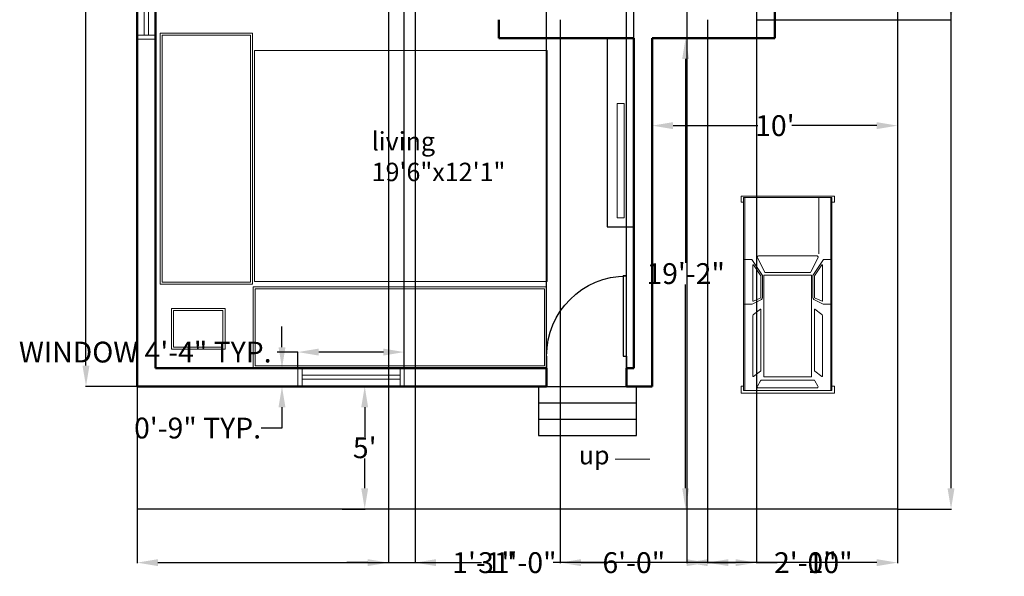
# Model space of a CAD drawing. Units: inches. Extents: x 20 to 3619, y 7 to 1288.
# Tile 1 of 4: x 3085 to 3567, y 695 to 967. Entities that reach past the tile are written whole.
import ezdxf

# ---------------------------------------------------------------- set-up
doc = ezdxf.new("R2010")
doc.units = ezdxf.units.IN
doc.header["$MEASUREMENT"] = 0
for name, color, linetype, lineweight in [('A-ANNO-DIMS', 2, 'Continuous', 18), ('A-ANNO-SYMB', 7, 'Continuous', 18), ('A-ANNO-TEXT', 7, 'Continuous', 18), ('A-AREA-IDEN', 7, 'Continuous', 25), ('A-DOOR', 3, 'Continuous', 25), ('A-FLOR-CASE', 9, 'Continuous', 25), ('A-FLOR-STRS', 7, 'Continuous', 25), ('A-FURN', 8, 'Continuous', 18), ('A-GLAZ', 4, 'Continuous', 18), ('A-SITE-VEHC', 8, 'Continuous', 13), ('A-WALL', 7, 'Continuous', 50), ('C-PROP', 8, 'Continuous', 25)]:
    doc.layers.add(name, color=color, linetype=linetype, lineweight=lineweight)
doc.styles.get("Standard").update_dxf_attribs({"font": 'arial.ttf'})
doc.dimstyles.get("Standard").update_dxf_attribs({"dimtxt": 10.18, "dimasz": 10.18, "dimexe": 0.18, "dimexo": 0.0625, "dimgap": 0.09, "dimtad": 0, "dimtih": 1, "dimtoh": 1, "dimdec": 0, "dimzin": 0, "dimdsep": 46, "dimlunit": 3, "dimtxsty": 'Standard', "dimcen": 0.09, "dimadec": 0, "dimazin": 0, "dimtfac": 1, "dimtdec": 0, "dimtofl": 0, "dimtmove": 0, "dimatfit": 3, "dimfxl": 1, "dimtolj": 1, "dimtzin": 0, "dimarcsym": 0})

# ---------------------------------------------------------------- blocks, each defined once
blk = doc.blocks.new('*U2')
for p, q in [((0, 0), (0, -6)), ((40, 0), (40, -6))]:
    blk.add_line(p, q)
blk.add_lwpolyline([(0, 0), (0, 40), (1.75, 40), (1.75, 0)], close=True)
blk.add_arc((0, 0), 40, 0, 90)
blk = doc.blocks.new('*D4')
at = {"layer": 'A-ANNO-DIMS', "color": 0, "lineweight": -2, "transparency": 16777216}
for p, q in [((3142.66, 1195.69), (3117.53, 1195.69)), ((3117.71, 1185.51), (3117.71, 996.98)), ((3117.71, 797.87), (3117.71, 986.4)), ((3142.66, 787.69), (3117.53, 787.69))]:
    blk.add_line(p, q, dxfattribs=at)
at = {"layer": 'A-ANNO-DIMS', "color": 0, "transparency": 16777216}
for points in [[(3116.01, 1185.51), (3119.4, 1185.51), (3117.71, 1195.69)], [(3116.01, 797.87), (3119.4, 797.87), (3117.71, 787.69)]]:
    blk.add_solid(points, dxfattribs=at)
at = {"layer": 'Defpoints', "color": 0, "transparency": 16777216}
for p in [(3117.71, 1195.69), (3142.72, 1195.69), (3142.72, 787.69)]:
    blk.add_point(p, dxfattribs=at)
at = {"layer": 'A-ANNO-DIMS', "color": 0, "transparency": 16777216, "insert": (3117.71, 991.69), "char_height": 10.18, "attachment_point": 5}
blk.add_mtext("\\A1;34'", dxfattribs=at)
blk = doc.blocks.new('*D6')
at = {"layer": 'A-ANNO-DIMS', "color": 0, "lineweight": -2, "transparency": 16777216}
for p, q in [((3394.72, 921.25), (3394.72, 915.08)), ((3514.72, 921.25), (3514.72, 915.08)), ((3404.9, 915.26), (3446.47, 915.26)), ((3504.54, 915.26), (3462.97, 915.26))]:
    blk.add_line(p, q, dxfattribs=at)
at = {"layer": 'A-ANNO-DIMS', "color": 0, "transparency": 16777216}
for points in [[(3404.9, 916.96), (3404.9, 913.56), (3394.72, 915.26)], [(3504.54, 916.96), (3504.54, 913.56), (3514.72, 915.26)]]:
    blk.add_solid(points, dxfattribs=at)
at = {"layer": 'Defpoints', "color": 0, "transparency": 16777216}
for p in [(3394.72, 921.31), (3514.72, 921.31), (3514.72, 915.26)]:
    blk.add_point(p, dxfattribs=at)
at = {"layer": 'A-ANNO-DIMS', "color": 0, "transparency": 16777216, "insert": (3454.72, 915.26), "char_height": 10.18, "attachment_point": 5}
blk.add_mtext("\\A1;10'", dxfattribs=at)
blk = doc.blocks.new('*D7')
at = {"layer": 'A-ANNO-DIMS', "color": 0, "lineweight": -2, "transparency": 16777216}
for p, q in [((3414.91, 958.08), (3410.9, 958.08)), ((3411.08, 947.9), (3411.08, 848.18)), ((3411.08, 737.87), (3411.08, 837.6)), ((3414.91, 727.69), (3410.9, 727.69))]:
    blk.add_line(p, q, dxfattribs=at)
at = {"layer": 'A-ANNO-DIMS', "color": 0, "transparency": 16777216}
for points in [[(3409.39, 947.9), (3412.78, 947.9), (3411.08, 958.08)], [(3409.39, 737.87), (3412.78, 737.87), (3411.08, 727.69)]]:
    blk.add_solid(points, dxfattribs=at)
at = {"layer": 'Defpoints', "color": 0, "transparency": 16777216}
for p in [(3414.97, 958.08), (3411.08, 727.69), (3414.97, 727.69)]:
    blk.add_point(p, dxfattribs=at)
at = {"layer": 'A-ANNO-DIMS', "color": 0, "transparency": 16777216, "insert": (3411.08, 842.89), "char_height": 10.18, "attachment_point": 5}
blk.add_mtext('\\A1;19\'-2"', dxfattribs=at)
blk = doc.blocks.new('*D8')
at = {"layer": 'A-ANNO-DIMS', "color": 0, "lineweight": -2, "transparency": 16777216}
for p, q in [((3242.96, 787.69), (3254.25, 787.69)), ((3254.07, 777.51), (3254.07, 762.96)), ((3254.07, 737.87), (3254.07, 752.43)), ((3242.96, 727.69), (3254.25, 727.69))]:
    blk.add_line(p, q, dxfattribs=at)
at = {"layer": 'A-ANNO-DIMS', "color": 0, "transparency": 16777216}
for points in [[(3252.37, 777.51), (3255.76, 777.51), (3254.07, 787.69)], [(3252.37, 737.87), (3255.76, 737.87), (3254.07, 727.69)]]:
    blk.add_solid(points, dxfattribs=at)
at = {"layer": 'Defpoints', "color": 0, "transparency": 16777216}
for p in [(3242.89, 787.69), (3242.89, 727.69), (3254.07, 727.69)]:
    blk.add_point(p, dxfattribs=at)
at = {"layer": 'A-ANNO-DIMS', "color": 0, "transparency": 16777216, "insert": (3254.07, 757.69), "char_height": 10.18, "attachment_point": 5}
blk.add_mtext("\\A1;5'", dxfattribs=at)
blk = doc.blocks.new('*U13')
for p, q in [((1.28, 38.87), (175.66, 38.87)), ((1.28, 28.15), (52.13, 28.15)), ((1.28, -28.15), (52.13, -28.15)), ((1.28, -38.87), (175.66, -38.87))]:
    blk.add_line(p, q)
for points in [[(5.57, 40.01), (5.57, 42.18), (0, 42.18), (0, -42.18), (5.57, -42.18), (5.57, -40.01), (1.28, -40.01), (1.28, 40.01)], [(1.28, 40.01), (175.66, 40.01), (175.66, -40.01), (1.28, -40.01)], [(171.74, 40.01), (175.66, 40.01), (175.66, -40.01), (171.74, -40.01), (171.74, -42.18), (178.14, -42.18), (178.14, 42.18), (171.74, 42.18)], [(71.47, 21.48), (163.42, 21.48), (163.42, -21.48), (71.47, -21.48)]]:
    blk.add_lwpolyline(points, close=True)
for points in [[(57.15, 40.01), (57.15, 32.39), (71.72, 22.83, 0.086577), (72.56, 22.68), (91.59, 22.68, 0.227875), (93.54, 23.62), (97.72, 32.11), (97.72, 40.01)], [(57.15, -40.01), (57.15, -32.39), (71.72, -22.83, -0.086577), (72.56, -22.68), (91.59, -22.68, -0.227875), (93.54, -23.62), (97.72, -32.11), (97.72, -40.01)]]:
    blk.add_lwpolyline(points, format="xyb")
for points in [[(55.49, 27.42), (68.59, 20.89, -0.284287), (69.14, 19.99), (69.14, -19.99, -0.284287), (68.59, -20.89), (55.49, -27.42, -0.557284), (54.05, -26.53), (54.05, 26.53, -0.557284)], [(62.08, 30.95), (72.14, 24.35, 0.146139), (72.69, 24.18), (91.42, 24.18, 0.29766), (92.33, 24.78), (95.09, 31.05, 0.541236), (94.86, 31.41), (62.21, 31.41, 0.744989)], [(102.19, 24.58), (106.97, 31, -0.236929), (107.78, 31.41), (162.91, 31.41, -0.621576), (163.11, 31), (158.19, 24.58, -0.233368), (157.39, 24.18), (102.39, 24.18, -0.616908)], [(171.88, 27.31), (166.83, 24.47, 0.271143), (166.32, 23.6), (166.32, -23.6, 0.271143), (166.83, -24.47), (171.88, -27.31, 0.573387), (173.37, -26.44), (173.37, 26.44, 0.573387)], [(62.08, -30.95), (72.14, -24.35, -0.146139), (72.69, -24.18), (91.42, -24.18, -0.29766), (92.33, -24.78), (95.09, -31.05, -0.541236), (94.86, -31.41), (62.21, -31.41, -0.744989)], [(102.19, -24.58), (106.97, -31, 0.236929), (107.78, -31.41), (162.91, -31.41, 0.621576), (163.11, -31), (158.19, -24.58, 0.233368), (157.39, -24.18), (102.39, -24.18, 0.616908)]]:
    blk.add_lwpolyline(points, format="xyb", close=True)
blk = doc.blocks.new('WIN-48IN-PLAN')
for p, q in [((0, 0), (0, 9)), ((2, 0), (2, 9)), ((2, 5.5), (50, 5.5)), ((50, 0), (50, 9)), ((52, 0), (52, 9)), ((2, 3.5), (50, 3.5))]:
    blk.add_line(p, q)
blk = doc.blocks.new('*D22')
at = {"layer": 'A-ANNO-DIMS', "color": 0, "lineweight": -2, "transparency": 16777216}
for p, q in [((3221.39, 804.49), (3211.21, 804.49)), ((3221.39, 796.76), (3221.39, 804.67)), ((3263.21, 804.49), (3231.57, 804.49)), ((3273.39, 796.76), (3273.39, 804.67))]:
    blk.add_line(p, q, dxfattribs=at)
at = {"layer": 'A-ANNO-DIMS', "color": 0, "transparency": 16777216}
for points in [[(3231.57, 806.19), (3231.57, 802.8), (3221.39, 804.49)], [(3263.21, 806.19), (3263.21, 802.8), (3273.39, 804.49)]]:
    blk.add_solid(points, dxfattribs=at)
at = {"layer": 'Defpoints', "color": 0, "transparency": 16777216}
for p in [(3221.39, 804.49), (3221.39, 796.69), (3273.39, 796.69)]:
    blk.add_point(p, dxfattribs=at)
at = {"layer": 'A-ANNO-DIMS', "color": 0, "transparency": 16777216, "insert": (3146.71, 804.49), "char_height": 10.18, "attachment_point": 5}
blk.add_mtext('\\A1;WINDOW 4\'-4" TYP.', dxfattribs=at)
blk = doc.blocks.new('*D23')
at = {"layer": 'A-ANNO-DIMS', "color": 0, "lineweight": -2, "transparency": 16777216}
for p, q in [((3213.59, 806.87), (3213.59, 817.05)), ((3221.33, 796.69), (3213.41, 796.69)), ((3221.33, 787.69), (3213.41, 787.69)), ((3213.59, 777.51), (3213.59, 767.33)), ((3213.59, 767.33), (3203.41, 767.33))]:
    blk.add_line(p, q, dxfattribs=at)
at = {"layer": 'A-ANNO-DIMS', "color": 0, "transparency": 16777216}
for points in [[(3211.9, 806.87), (3215.29, 806.87), (3213.59, 796.69)], [(3211.9, 777.51), (3215.29, 777.51), (3213.59, 787.69)]]:
    blk.add_solid(points, dxfattribs=at)
at = {"layer": 'Defpoints', "color": 0, "transparency": 16777216}
for p in [(3221.39, 796.69), (3213.59, 787.69), (3221.39, 787.69)]:
    blk.add_point(p, dxfattribs=at)
at = {"layer": 'A-ANNO-DIMS', "color": 0, "transparency": 16777216, "insert": (3172.3, 767.33), "char_height": 10.18, "attachment_point": 5}
blk.add_mtext('\\A1;0\'-9" TYP.', dxfattribs=at)
blk = doc.blocks.new('*D28')
at = {"layer": 'A-ANNO-DIMS', "color": 0, "lineweight": -2, "transparency": 16777216}
for p, q in [((3163.42, 1000.64), (3163.42, 991.78)), ((3221.69, 1000.64), (3221.69, 991.78)), ((3173.6, 991.96), (3211.51, 991.96)), ((3221.69, 991.96), (3231.87, 991.96))]:
    blk.add_line(p, q, dxfattribs=at)
at = {"layer": 'A-ANNO-DIMS', "color": 0, "transparency": 16777216}
for points in [[(3173.6, 993.66), (3173.6, 990.26), (3163.42, 991.96)], [(3211.51, 993.66), (3211.51, 990.26), (3221.69, 991.96)]]:
    blk.add_solid(points, dxfattribs=at)
at = {"layer": 'Defpoints', "color": 0, "transparency": 16777216}
for p in [(3163.42, 1000.7), (3221.69, 1000.7), (3221.69, 991.96)]:
    blk.add_point(p, dxfattribs=at)
at = {"layer": 'A-ANNO-DIMS', "color": 0, "transparency": 16777216, "insert": (3303.72, 991.96), "char_height": 10.18, "attachment_point": 5}
blk.add_mtext('\\A1;DINING SET 4\'-10 1/2"', dxfattribs=at)
blk = doc.blocks.new('*D36')
at = {"layer": 'A-ANNO-DIMS', "color": 0, "lineweight": -2, "transparency": 16777216}
for p, q in [((3142.72, 727.63), (3142.72, 701.31)), ((3514.72, 727.63), (3514.72, 701.31)), ((3152.9, 701.49), (3311.15, 701.49)), ((3504.54, 701.49), (3346.29, 701.49))]:
    blk.add_line(p, q, dxfattribs=at)
at = {"layer": 'A-ANNO-DIMS', "color": 0, "transparency": 16777216}
for points in [[(3152.9, 703.19), (3152.9, 699.8), (3142.72, 701.49)], [(3504.54, 703.19), (3504.54, 699.8), (3514.72, 701.49)]]:
    blk.add_solid(points, dxfattribs=at)
at = {"layer": 'Defpoints', "color": 0, "transparency": 16777216}
for p in [(3142.72, 727.69), (3514.72, 727.69), (3514.72, 701.49)]:
    blk.add_point(p, dxfattribs=at)
at = {"layer": 'A-ANNO-DIMS', "color": 0, "transparency": 16777216, "insert": (3328.72, 701.49), "char_height": 10.18, "attachment_point": 5}
blk.add_mtext('\\A1;31\'-0"', dxfattribs=at)
blk = doc.blocks.new('*D37')
at = {"layer": 'A-ANNO-DIMS', "color": 0, "lineweight": -2, "transparency": 16777216}
for p, q in [((3514.78, 1243.69), (3541.1, 1243.69)), ((3540.92, 1233.51), (3540.92, 990.98)), ((3540.92, 737.87), (3540.92, 980.4)), ((3514.78, 727.69), (3541.1, 727.69))]:
    blk.add_line(p, q, dxfattribs=at)
at = {"layer": 'A-ANNO-DIMS', "color": 0, "transparency": 16777216}
for points in [[(3539.22, 1233.51), (3542.61, 1233.51), (3540.92, 1243.69)], [(3539.22, 737.87), (3542.61, 737.87), (3540.92, 727.69)]]:
    blk.add_solid(points, dxfattribs=at)
at = {"layer": 'Defpoints', "color": 0, "transparency": 16777216}
for p in [(3514.72, 1243.69), (3540.92, 1243.69), (3514.72, 727.69)]:
    blk.add_point(p, dxfattribs=at)
at = {"layer": 'A-ANNO-DIMS', "color": 0, "transparency": 16777216, "insert": (3540.92, 985.69), "char_height": 10.18, "attachment_point": 5}
blk.add_mtext('\\A1;43\'-0"', dxfattribs=at)
blk = doc.blocks.new('*D40')
at = {"layer": 'A-ANNO-DIMS', "color": 0, "lineweight": -2, "transparency": 16777216}
for p, q in [((3332.89, 1272.89), (3322.71, 1272.89)), ((3343.07, 796.76), (3343.07, 1273.07)), ((3382.22, 796.76), (3382.22, 1273.07)), ((3392.4, 1272.89), (3402.58, 1272.89))]:
    blk.add_line(p, q, dxfattribs=at)
at = {"layer": 'A-ANNO-DIMS', "color": 0, "transparency": 16777216}
for points in [[(3332.89, 1274.59), (3332.89, 1271.2), (3343.07, 1272.89)], [(3392.4, 1274.59), (3392.4, 1271.2), (3382.22, 1272.89)]]:
    blk.add_solid(points, dxfattribs=at)
at = {"layer": 'Defpoints', "color": 0, "transparency": 16777216}
for p in [(3382.22, 1272.89), (3343.07, 796.69), (3382.22, 796.69)]:
    blk.add_point(p, dxfattribs=at)
at = {"layer": 'A-ANNO-DIMS', "color": 0, "transparency": 16777216, "insert": (3362.64, 1272.89), "char_height": 10.18, "attachment_point": 5}
blk.add_mtext('\\A1;3\'-3"', dxfattribs=at)
blk = doc.blocks.new('*D41')
at = {"layer": 'A-ANNO-DIMS', "color": 0, "lineweight": -2, "transparency": 16777216}
for p, q in [((3263.21, 1272.89), (3253.03, 1272.89)), ((3273.39, 796.76), (3273.39, 1273.07)), ((3343.07, 796.76), (3343.07, 1273.07)), ((3353.25, 1272.89), (3363.43, 1272.89))]:
    blk.add_line(p, q, dxfattribs=at)
at = {"layer": 'A-ANNO-DIMS', "color": 0, "transparency": 16777216}
for points in [[(3263.21, 1274.59), (3263.21, 1271.2), (3273.39, 1272.89)], [(3353.25, 1274.59), (3353.25, 1271.2), (3343.07, 1272.89)]]:
    blk.add_solid(points, dxfattribs=at)
at = {"layer": 'Defpoints', "color": 0, "transparency": 16777216}
for p in [(3343.07, 1272.89), (3273.39, 796.69), (3343.07, 796.69)]:
    blk.add_point(p, dxfattribs=at)
at = {"layer": 'A-ANNO-DIMS', "color": 0, "transparency": 16777216, "insert": (3308.23, 1272.89), "char_height": 10.18, "attachment_point": 5}
blk.add_mtext('\\A1;5\'-9 1/2"', dxfattribs=at)
blk = doc.blocks.new('*D42')
at = {"layer": 'A-ANNO-DIMS', "color": 0, "lineweight": -2, "transparency": 16777216}
for p, q in [((3372.04, 1272.89), (3361.86, 1272.89)), ((3382.22, 796.76), (3382.22, 1273.07)), ((3385.72, 796.76), (3385.72, 1273.07)), ((3395.9, 1272.89), (3406.08, 1272.89))]:
    blk.add_line(p, q, dxfattribs=at)
at = {"layer": 'A-ANNO-DIMS', "color": 0, "transparency": 16777216}
for points in [[(3372.04, 1274.59), (3372.04, 1271.2), (3382.22, 1272.89)], [(3395.9, 1274.59), (3395.9, 1271.2), (3385.72, 1272.89)]]:
    blk.add_solid(points, dxfattribs=at)
at = {"layer": 'Defpoints', "color": 0, "transparency": 16777216}
for p in [(3385.72, 1272.89), (3382.22, 796.69), (3385.72, 796.69)]:
    blk.add_point(p, dxfattribs=at)
at = {"layer": 'A-ANNO-DIMS', "color": 0, "transparency": 16777216, "insert": (3431.56, 1272.89), "char_height": 10.18, "attachment_point": 5}
blk.add_mtext('\\A1;0\'-3 1/2"', dxfattribs=at)
blk = doc.blocks.new('*D45')
at = {"layer": 'A-ANNO-DIMS', "color": 0, "lineweight": -2, "transparency": 16777216}
for p, q in [((3411.72, 1186.63), (3411.72, 701.31)), ((3445.72, 1186.63), (3445.72, 701.31)), ((3421.9, 701.49), (3435.54, 701.49)), ((3445.72, 701.49), (3455.9, 701.49))]:
    blk.add_line(p, q, dxfattribs=at)
at = {"layer": 'A-ANNO-DIMS', "color": 0, "transparency": 16777216}
for points in [[(3421.9, 703.19), (3421.9, 699.8), (3411.72, 701.49)], [(3435.54, 703.19), (3435.54, 699.8), (3445.72, 701.49)]]:
    blk.add_solid(points, dxfattribs=at)
at = {"layer": 'Defpoints', "color": 0, "transparency": 16777216}
for p in [(3411.72, 1186.69), (3445.72, 1186.69), (3445.72, 701.49)]:
    blk.add_point(p, dxfattribs=at)
at = {"layer": 'A-ANNO-DIMS', "color": 0, "transparency": 16777216, "insert": (3473.56, 701.49), "char_height": 10.18, "attachment_point": 5}
blk.add_mtext('\\A1;2\'-10"', dxfattribs=at)
blk = doc.blocks.new('*D47')
at = {"layer": 'A-ANNO-DIMS', "color": 0, "lineweight": -2, "transparency": 16777216}
for p, q in [((3265.72, 1186.63), (3265.72, 701.31)), ((3278.72, 1186.63), (3278.72, 701.31)), ((3255.54, 701.49), (3245.36, 701.49)), ((3288.9, 701.49), (3299.08, 701.49))]:
    blk.add_line(p, q, dxfattribs=at)
at = {"layer": 'A-ANNO-DIMS', "color": 0, "transparency": 16777216}
for points in [[(3255.54, 703.19), (3255.54, 699.8), (3265.72, 701.49)], [(3288.9, 703.19), (3288.9, 699.8), (3278.72, 701.49)]]:
    blk.add_solid(points, dxfattribs=at)
at = {"layer": 'Defpoints', "color": 0, "transparency": 16777216}
for p in [(3265.72, 1186.69), (3278.72, 1186.69), (3278.72, 701.49)]:
    blk.add_point(p, dxfattribs=at)
at = {"layer": 'A-ANNO-DIMS', "color": 0, "transparency": 16777216, "insert": (3312.22, 701.49), "char_height": 10.18, "attachment_point": 5}
blk.add_mtext('\\A1;1\'-1"', dxfattribs=at)
blk = doc.blocks.new('*D49')
at = {"layer": 'A-ANNO-DIMS', "color": 0, "lineweight": -2, "transparency": 16777216}
for p, q in [((3349.72, 967.02), (3349.72, 701.31)), ((3421.72, 967.02), (3421.72, 701.31)), ((3359.9, 701.49), (3372.07, 701.49)), ((3411.54, 701.49), (3399.37, 701.49))]:
    blk.add_line(p, q, dxfattribs=at)
at = {"layer": 'A-ANNO-DIMS', "color": 0, "transparency": 16777216}
for points in [[(3359.9, 703.19), (3359.9, 699.8), (3349.72, 701.49)], [(3411.54, 703.19), (3411.54, 699.8), (3421.72, 701.49)]]:
    blk.add_solid(points, dxfattribs=at)
at = {"layer": 'Defpoints', "color": 0, "transparency": 16777216}
for p in [(3349.72, 967.08), (3421.72, 967.08), (3421.72, 701.49)]:
    blk.add_point(p, dxfattribs=at)
at = {"layer": 'A-ANNO-DIMS', "color": 0, "transparency": 16777216, "insert": (3385.72, 701.49), "char_height": 10.18, "attachment_point": 5}
blk.add_mtext('\\A1;6\'-0"', dxfattribs=at)
blk = doc.blocks.new('*D50')
at = {"layer": 'A-ANNO-DIMS', "color": 0, "lineweight": -2, "transparency": 16777216}
for p, q in [((3421.72, 967.02), (3421.72, 701.31)), ((3445.72, 967.02), (3445.72, 701.31)), ((3431.9, 701.49), (3435.54, 701.49)), ((3445.72, 701.49), (3455.9, 701.49))]:
    blk.add_line(p, q, dxfattribs=at)
at = {"layer": 'A-ANNO-DIMS', "color": 0, "transparency": 16777216}
for points in [[(3431.9, 703.19), (3431.9, 699.8), (3421.72, 701.49)], [(3435.54, 703.19), (3435.54, 699.8), (3445.72, 701.49)]]:
    blk.add_solid(points, dxfattribs=at)
at = {"layer": 'Defpoints', "color": 0, "transparency": 16777216}
for p in [(3421.72, 967.08), (3445.72, 967.08), (3445.72, 701.49)]:
    blk.add_point(p, dxfattribs=at)
at = {"layer": 'A-ANNO-DIMS', "color": 0, "transparency": 16777216, "insert": (3469.61, 701.49), "char_height": 10.18, "attachment_point": 5}
blk.add_mtext('\\A1;2\'-0"', dxfattribs=at)
blk = doc.blocks.new('*D51')
at = {"layer": 'A-ANNO-DIMS', "color": 0, "lineweight": -2, "transparency": 16777216}
for p, q in [((3445.78, 1012.69), (3541.1, 1012.69)), ((3540.92, 1002.51), (3540.92, 995.25)), ((3540.92, 977.26), (3540.92, 984.53)), ((3445.78, 967.08), (3541.1, 967.08))]:
    blk.add_line(p, q, dxfattribs=at)
at = {"layer": 'A-ANNO-DIMS', "color": 0, "transparency": 16777216}
for points in [[(3539.22, 1002.51), (3542.61, 1002.51), (3540.92, 1012.69)], [(3539.22, 977.26), (3542.61, 977.26), (3540.92, 967.08)]]:
    blk.add_solid(points, dxfattribs=at)
at = {"layer": 'Defpoints', "color": 0, "transparency": 16777216}
for p in [(3445.72, 1012.69), (3540.92, 1012.69), (3445.72, 967.08)]:
    blk.add_point(p, dxfattribs=at)
at = {"layer": 'A-ANNO-DIMS', "color": 0, "transparency": 16777216, "insert": (3540.92, 989.89), "char_height": 10.18, "attachment_point": 5}
blk.add_mtext('\\A1;3\'-9 1/2"', dxfattribs=at)

msp = doc.modelspace()

# ---------------------------------------------------------------- linework, layer by layer
at = {"layer": 'A-ANNO-SYMB'}
msp.add_line((3376.65, 752.17), (3393.53, 752.17), dxfattribs=at)
at = {"layer": 'A-FLOR-CASE'}
for p, q in [((3372.71, 958.08), (3372.71, 865.76)), ((3372.71, 865.76), (3385.72, 865.76))]:
    msp.add_line(p, q, dxfattribs=at)
at = {"layer": 'A-FLOR-STRS'}
for p, q in [((3339.06, 787.69), (3339.06, 763.69)), ((3343.07, 787.69), (3382.22, 787.69)), ((3387.1, 763.69), (3387.1, 787.69)), ((3339.06, 779.69), (3387.1, 779.69)), ((3339.06, 771.69), (3387.1, 771.69)), ((3339.06, 763.69), (3387.1, 763.69)), ((3343.07, 763.69), (3382.22, 763.69))]:
    msp.add_line(p, q, dxfattribs=at)
at = {"layer": 'A-FURN'}
for p, q in [((3200.16, 952.02), (3200.16, 839.02)), ((3343.41, 952.02), (3200.16, 952.02)), ((3343.41, 839.02), (3343.41, 952.02)), ((3200.16, 839.02), (3343.41, 839.02))]:
    msp.add_line(p, q, dxfattribs=at)
for points in [[(3199.16, 960.47), (3154.04, 960.47), (3154.04, 837.69), (3199.16, 837.69)], [(3198.16, 959.47), (3155.04, 959.47), (3155.04, 838.69), (3198.16, 838.69)], [(3381.02, 926.02), (3377.64, 926.02), (3377.64, 870.19), (3381.02, 870.19)], [(3343.07, 796.69), (3199.46, 796.69), (3199.46, 836.48), (3343.07, 836.48)], [(3342.07, 797.69), (3200.46, 797.69), (3200.46, 835.48), (3342.07, 835.48)], [(3159.58, 825.78), (3185.73, 825.78), (3185.73, 805.89), (3159.58, 805.89)], [(3160.58, 824.78), (3184.73, 824.78), (3184.73, 806.89), (3160.58, 806.89)]]:
    msp.add_lwpolyline(points, close=True, dxfattribs=at)
at = {"layer": 'A-GLAZ'}
msp.add_line((3148.22, 1007.59), (3148.22, 959.59), dxfattribs=at)
at = {"layer": 'A-WALL'}
for p, q in [((3142.72, 787.69), (3142.72, 1195.69)), ((3454.72, 1195.69), (3454.72, 958.08)), ((3151.72, 796.69), (3151.72, 1078.69)), ((3319.72, 958.08), (3319.72, 967.08)), ((3385.72, 958.08), (3319.72, 958.08)), ((3385.72, 958.08), (3385.72, 796.69)), ((3454.72, 958.08), (3394.72, 958.08)), ((3394.72, 958.08), (3394.72, 787.69)), ((3343.07, 796.69), (3151.72, 796.69)), ((3343.07, 796.69), (3343.07, 787.69)), ((3385.72, 796.69), (3382.22, 796.69)), ((3382.22, 796.69), (3382.22, 787.69)), ((3343.07, 787.69), (3142.72, 787.69)), ((3394.72, 787.69), (3382.22, 787.69))]:
    msp.add_line(p, q, dxfattribs=at)
at = {"layer": 'C-PROP'}
for p, q in [((3514.72, 1243.69), (3514.72, 727.69)), ((3142.72, 787.69), (3142.72, 727.69)), ((3514.72, 727.69), (3142.72, 727.69))]:
    msp.add_line(p, q, dxfattribs=at)

# ---------------------------------------------------------------- block references
at = {"layer": 'A-DOOR', "xscale": -0.9786925292065342, "yscale": 0.9786925292065342, "zscale": 0.9786925292065342}
msp.add_blockref('*U2', (3382.22, 802.57), dxfattribs=at)
at = {"layer": 'A-GLAZ'}
for p, rotation in [((3151.72, 957.59), 89.99999999999845), ((3273.39, 796.69), 180)]:
    msp.add_blockref('WIN-48IN-PLAN', p, dxfattribs=dict(at, rotation=rotation))
at = {"layer": 'A-SITE-VEHC', "xscale": 0.5411640969772729, "yscale": 0.5411640969772729, "zscale": 0.5411640969772729, "rotation": 270}
msp.add_blockref('*U13', (3461, 880.79), dxfattribs=at)

# ---------------------------------------------------------------- texts
at = {"layer": 'A-ANNO-TEXT', "insert": (3358.79, 758.57), "char_height": 9, "attachment_point": 1}
msp.add_mtext_dynamic_manual_height_columns('up ', width=17.3739, gutter_width=1, heights=[0], dxfattribs=at)
at = {"layer": 'A-AREA-IDEN', "insert": (3257.44, 912.11), "char_height": 9, "attachment_point": 1}
msp.add_mtext_dynamic_manual_height_columns('living \\P19\'6"x12\'1" ', width=17.3739, gutter_width=1, heights=[0], dxfattribs=at)

# ---------------------------------------------------------------- dimensions: what is measured, and where the dimension line sits
at = {"layer": 'A-ANNO-DIMS'}
for base, p1, p2, override, picture, middle in [((3343.07, 1272.89), (3273.39, 796.69), (3343.07, 796.69), {"dimdec": 1, "dimlfac": 1, "dimrnd": 0, "dimzin": 1, "dimdsep": 46, "dimlunit": 4, "dimfrac": 2}, '*D41', (3308.23, 1272.89)), ((3385.72, 1272.89), (3382.22, 796.69), (3385.72, 796.69), {"dimdec": 1, "dimlfac": 1, "dimrnd": 0, "dimzin": 1, "dimdsep": 46, "dimlunit": 4, "dimfrac": 2}, '*D42', (3431.56, 1272.89)), ((3382.2188, 1272.8933), (3343.0711, 796.6933), (3382.2188, 796.6933), {"dimdec": 1, "dimlfac": 1, "dimrnd": 0, "dimzin": 1, "dimdsep": 46, "dimlunit": 4, "dimfrac": 2}, '*D40', (3362.6449, 1272.8933)), ((3278.72, 701.49), (3265.72, 1186.69), (3278.72, 1186.69), {"dimdec": 1, "dimlfac": 1, "dimrnd": 0, "dimzin": 1, "dimdsep": 46, "dimlunit": 4, "dimfrac": 2}, '*D47', (3312.22, 701.49)), ((3445.72, 701.49), (3411.72, 1186.69), (3445.72, 1186.69), {"dimdec": 1, "dimlfac": 1, "dimrnd": 0, "dimzin": 1, "dimdsep": 46, "dimlunit": 4, "dimfrac": 2}, '*D45', (3473.56, 701.49)), ((3421.72, 701.49), (3349.72, 967.08), (3421.72, 967.08), {"dimdec": 1, "dimlfac": 1, "dimrnd": 0, "dimzin": 1, "dimdsep": 46, "dimlunit": 4, "dimfrac": 2}, '*D49', (3385.72, 701.49)), ((3445.72, 701.49), (3421.72, 967.08), (3445.72, 967.08), {"dimdec": 1, "dimlfac": 1, "dimrnd": 0, "dimzin": 1, "dimdsep": 46, "dimlunit": 4, "dimfrac": 2}, '*D50', (3469.61, 701.49)), ((3514.72, 915.26), (3394.72, 921.31), (3514.72, 921.31), {"dimclrd": 0, "dimclre": 0, "dimclrt": 0}, '*D6', (3454.72, 915.26)), ((3514.72, 701.49), (3142.72, 727.69), (3514.72, 727.69), {"dimdec": 1, "dimlfac": 1, "dimrnd": 0, "dimzin": 1, "dimdsep": 46, "dimlunit": 4, "dimfrac": 2}, '*D36', (3328.72, 701.49))]:
    dim = msp.add_linear_dim(base=base, p1=p1, p2=p2, dimstyle='Standard', override=override, dxfattribs=at)
    dim.commit()
    dim.dimension.update_dxf_attribs({"geometry": picture, "text_midpoint": middle})
for base, p1, p2, override, picture, middle in [((3540.92, 1243.69), (3514.72, 727.69), (3514.72, 1243.69), {"dimdec": 1, "dimlfac": 1, "dimrnd": 0, "dimzin": 1, "dimdsep": 46, "dimlunit": 4, "dimfrac": 2}, '*D37', (3540.92, 985.69)), ((3117.71, 1195.69), (3142.72, 787.69), (3142.72, 1195.69), {"dimclrd": 0, "dimclre": 0, "dimclrt": 0}, '*D4', (3117.71, 991.69)), ((3540.92, 1012.69), (3445.72, 967.08), (3445.72, 1012.69), {"dimdec": 1, "dimlfac": 1, "dimrnd": 0, "dimzin": 1, "dimdsep": 46, "dimlunit": 4, "dimfrac": 2}, '*D51', (3540.92, 989.89)), ((3411.08, 727.69), (3414.97, 958.08), (3414.97, 727.69), {"dimclrd": 0, "dimclre": 0, "dimclrt": 0}, '*D7', (3411.08, 842.89)), ((3254.07, 727.69), (3242.89, 787.69), (3242.89, 727.69), {"dimclrd": 0, "dimclre": 0, "dimclrt": 0}, '*D8', (3254.07, 757.69))]:
    dim = msp.add_linear_dim(base=base, p1=p1, p2=p2, angle=90, dimstyle='Standard', override=override, dxfattribs=at)
    dim.commit()
    dim.dimension.update_dxf_attribs({"geometry": picture, "text_midpoint": middle})
dim = msp.add_linear_dim(base=(3221.69, 991.96), p1=(3163.42, 1000.7), p2=(3221.69, 1000.7), text='DINING SET <>', dimstyle='Standard', override={"dimdec": 1, "dimlfac": 1, "dimrnd": 0, "dimzin": 1, "dimdsep": 46, "dimlunit": 4, "dimfrac": 2}, dxfattribs=at)
dim.commit()
dim.dimension.update_dxf_attribs({"geometry": '*D28', "text_midpoint": (3303.72, 991.96)})
for base, p1, p2, angle, text, picture, middle in [((3221.39, 804.49), (3273.39, 796.69), (3221.39, 796.69), 180, 'WINDOW <> TYP.', '*D22', (3146.71, 804.49)), ((3213.59, 787.69), (3221.39, 796.69), (3221.39, 787.69), 270, '<> TYP.', '*D23', (3172.3, 767.33))]:
    dim = msp.add_linear_dim(base=base, p1=p1, p2=p2, angle=angle, text=text, dimstyle='Standard', override={"dimdec": 1, "dimlfac": 1, "dimrnd": 0, "dimzin": 1, "dimdsep": 46, "dimlunit": 4, "dimfrac": 2}, dxfattribs=at)
    dim.commit()
    dim.dimension.update_dxf_attribs({"geometry": picture, "text_midpoint": middle})

doc.saveas('drawing.dxf')
